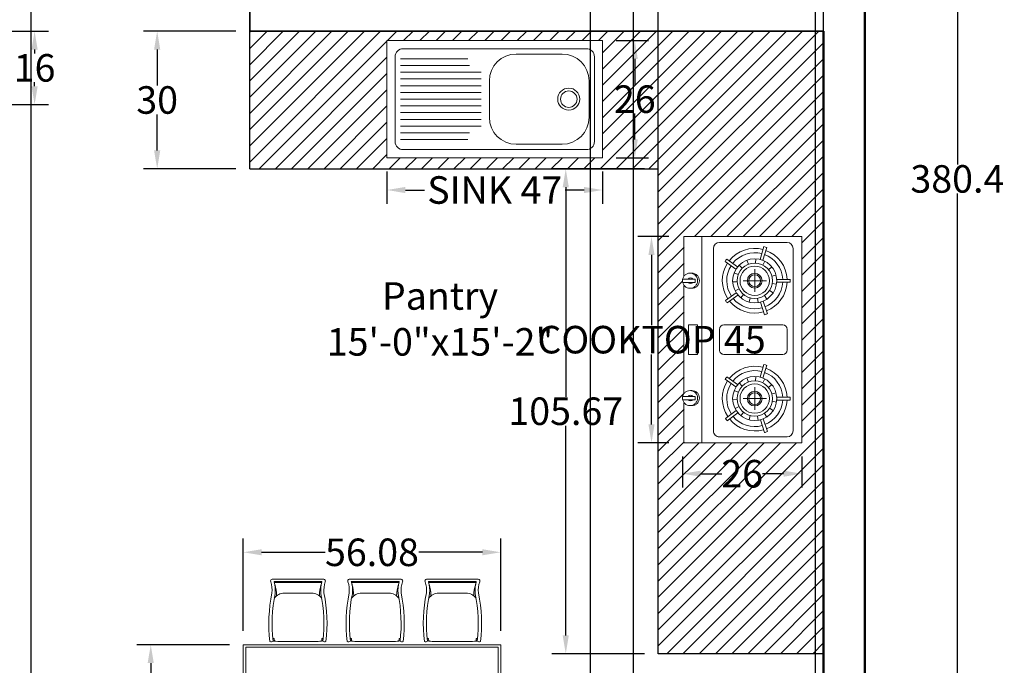
# Model space of a CAD drawing. Units: inches. Extents: x 89 to 490, y -59 to 378.
# Tile 18 of 20: x 275 to 490, y 58 to 198. Entities that reach past the tile are written whole.
import ezdxf

# ---------------------------------------------------------------- set-up
doc = ezdxf.new("R2010")
doc.units = ezdxf.units.IN
doc.header["$MEASUREMENT"] = 0
for name, color, linetype, lineweight in [('A-ANNO-DIMS', 2, 'Continuous', 18), ('A-AREA-IDEN', 7, 'Continuous', 18), ('A-FLOR-CASE', 21, 'Continuous', 25), ('A-FLOR-CASE-PATT', 25, 'Continuous', 13), ('Dining Table', 155, 'Continuous', 18), ('Gas Stove', 51, 'Continuous', 18), ('Inner Walls', 31, 'Continuous', 35), ('Outer Walls', 12, 'Continuous', 50), ('Sink', 21, 'Continuous', 18)]:
    doc.layers.add(name, color=color, linetype=linetype, lineweight=lineweight)
doc.styles.get("Standard").update_dxf_attribs({"font": 'arial.ttf'})
doc.dimstyles.get("Standard").update_dxf_attribs({"dimtxt": 6, "dimasz": 4, "dimexe": 3, "dimexo": 3, "dimgap": 0.09, "dimtad": 0, "dimtih": 1, "dimtoh": 1, "dimdec": 1, "dimzin": 0, "dimdsep": 46, "dimlunit": 3, "dimtxsty": 'Standard', "dimcen": 0.09, "dimadec": 0, "dimazin": 0, "dimtfac": 1, "dimtdec": 1, "dimtofl": 0, "dimtmove": 0, "dimatfit": 3, "dimfxl": 1, "dimtolj": 1, "dimtzin": 0, "dimarcsym": 0})

# ---------------------------------------------------------------- blocks, each defined once
blk = doc.blocks.new('A$C51F1')
at = {"color": 0}
for p, q in [((0.2273, 0.4758), (0.0436, 0.4758)), ((0.2273, 0.4676), (0.0439, 0.4676)), ((0.2273, 0.4668), (0.0439, 0.4668)), ((0.2273, 0.4758), (0.4111, 0.4758)), ((0.2273, 0.4676), (0.4107, 0.4676)), ((0.2273, 0.4668), (0.4107, 0.4668)), ((0.2273, 0.3858), (0.1205, 0.3858)), ((0.2273, 0.3858), (0.3341, 0.3858)), ((0.0417, 0.0321), (0.0321, 0.0321)), ((0.0417, 0.0321), (0.0326, 0.0278)), ((0.0435, 0.0127), (0.0417, 0.0321)), ((0.4112, 0.0127), (0.4129, 0.0321)), ((0.4129, 0.0321), (0.4225, 0.0321)), ((0.4129, 0.0321), (0.4221, 0.0278))]:
    blk.add_line(p, q, dxfattribs=at)
blk.add_lwpolyline([(0.4387, 0.4737, 0.102523), (0.4291, 0.3863, -0.080461), (0.4447, 0.0091, -0.3023), (0.4203, 0.012, 0.197932), (0.4111, 0.0127, -0.028193), (0.3571, 0.0091), (0.227, 0.0091), (0.097, 0.0091, -0.028193), (0.0429, 0.0127, 0.197932), (0.0338, 0.012, -0.3023), (0.0093, 0.0091, -0.080461), (0.0249, 0.3863, 0.102523), (0.0153, 0.4737, -0.587111), (0.0261, 0.4929), (0.4279, 0.4929, -0.587111)], format="xyb", close=True, dxfattribs=at)
for centre, radius, start, end in [((0.044, 0.4735), 0.00242, 100.34496, 201.37417), ((-0.1898, 0.4063), 0.2409, 354.55133, 15.96258), ((0.0439, 0.4669), 0.000725, 87.37617, 197.52085), ((0.0438, 0.4664), 0.000433, 71.7715, 189.22024), ((0.6445, 0.4063), 0.2409, 164.03742, 185.44867), ((0.4107, 0.4669), 0.000725, 342.47915, 92.62383), ((0.4109, 0.4664), 0.000433, 350.77976, 108.2285), ((0.4106, 0.4735), 0.00242, 338.62583, 79.65504), ((0.1214, 0.2879), 0.0978, 90.51639, 143.19267), ((-0.2563, 0.3584), 0.3173, 1.15909, 17.56409), ((0.3332, 0.2879), 0.0978, 36.80733, 89.48361), ((0.7109, 0.3584), 0.3173, 162.43591, 178.84091), ((1.1806, 0.1494), 1.1544, 168.43567, 186.83625), ((-0.7259, 0.1494), 1.1544, 353.16375, 11.56433), ((0.0397, 0.0013), 0.012, 71.75361, 116.5375), ((0.4149, 0.0013), 0.012, 63.4625, 108.24639)]:
    blk.add_arc(centre, radius, start, end, dxfattribs=at)
blk = doc.blocks.new('A$C56104318')
for p, q in [((0, 0.609), (1.12, 0.609)), ((0, 0.609), (0, 0)), ((0.084, 0.567), (1.036, 0.567)), ((1.12, 0.609), (1.12, 0)), ((0.042, 0.525), (0.042, 0.084)), ((0.42, 0.5145), (0.07, 0.5145)), ((0.672, 0.539), (0.91, 0.539)), ((1.078, 0.525), (1.078, 0.084)), ((0.07, 0.4795), (0.4294, 0.4795)), ((0.07, 0.4445), (0.49, 0.4445)), ((0.07, 0.4095), (0.49, 0.4095)), ((0.07, 0.3745), (0.49, 0.3745)), ((0.532, 0.21), (0.532, 0.399)), ((1.05, 0.399), (1.05, 0.21)), ((0.07, 0.3395), (0.49, 0.3395)), ((0.07, 0.3045), (0.49, 0.3045)), ((0.07, 0.2695), (0.49, 0.2695)), ((0.07, 0.2345), (0.49, 0.2345)), ((0.07, 0.1995), (0.49, 0.1995)), ((0.07, 0.1645), (0.4898, 0.1645)), ((0.07, 0.1295), (0.4294, 0.1295)), ((0.07, 0.0945), (0.42, 0.0945)), ((0.91, 0.07), (0.672, 0.07)), ((1.036, 0.042), (0.084, 0.042)), ((1.12, 0), (0, 0))]:
    blk.add_line(p, q)
for radius in [0.0574, 0.0427]:
    blk.add_circle((0.945, 0.3045), radius)
for centre, radius, start, end in [((0.084, 0.525), 0.042, 90, 180), ((1.036, 0.525), 0.042, 0, 90), ((0.672, 0.399), 0.14, 90, 180), ((0.91, 0.399), 0.14, 0, 90), ((0.672, 0.21), 0.14, 180, 270), ((0.91, 0.21), 0.14, 270, 0), ((0.084, 0.084), 0.042, 180, 270), ((1.036, 0.084), 0.042, 270, 0)]:
    blk.add_arc(centre, radius, start, end)
blk = doc.blocks.new('A$C559B0E78')
at = {"xscale": 729, "yscale": 729, "zscale": 729}
blk.add_blockref('A$C56104318', (0, 0), dxfattribs=at)
blk = doc.blocks.new('Gas Stove')
at = {"color": 0}
for p, q in [((732.13, 198.42), (732.13, 184.15)), ((732.13, 198.42), (757.09, 198.42)), ((757.09, 198.42), (757.09, 184.15)), ((732.84, 196.63), (732.84, 188.43)), ((733.55, 197.35), (755.66, 197.35)), ((737.3, 195.38), (737.3, 196.99)), ((737.65, 195.38), (737.65, 196.99)), ((743.36, 196.63), (745.85, 196.63)), ((751.56, 195.38), (751.56, 196.99)), ((751.92, 195.38), (751.92, 196.99)), ((756.37, 196.63), (756.37, 188.43)), ((742.82, 196.1), (742.82, 188.97)), ((746.39, 196.1), (746.39, 188.97)), ((735.79, 194.79), (736.13, 194.37)), ((736.78, 195.3), (736.92, 194.78)), ((737.89, 195.35), (737.81, 194.83)), ((738.93, 194.96), (738.64, 194.51)), ((741.48, 194.24), (739.95, 193.73)), ((750.05, 194.79), (750.39, 194.37)), ((751.05, 195.3), (751.18, 194.78)), ((752.16, 195.35), (752.07, 194.83)), ((753.19, 194.96), (752.9, 194.51)), ((755.74, 194.24), (754.21, 193.73)), ((733.34, 193.83), (734.88, 193.35)), ((733.45, 194.17), (734.98, 193.69)), ((735.09, 193.93), (735.57, 193.68)), ((737.47, 194.12), (737.47, 191.3)), ((739.72, 194.17), (739.27, 193.88)), ((740.12, 193.13), (739.59, 193.05)), ((741.59, 193.9), (740.06, 193.39)), ((747.6, 193.83), (749.14, 193.35)), ((747.71, 194.17), (749.25, 193.69)), ((749.35, 193.93), (749.83, 193.68)), ((751.74, 194.12), (751.74, 191.3)), ((753.98, 194.17), (753.53, 193.88)), ((754.38, 193.13), (753.85, 193.05)), ((755.85, 193.9), (754.33, 193.39)), ((734.8, 192.85), (735.34, 192.82)), ((734.98, 191.75), (735.48, 191.95)), ((736.06, 192.71), (738.83, 192.71)), ((740.06, 192.02), (739.54, 192.16)), ((749.07, 192.85), (749.6, 192.82)), ((749.24, 191.75), (749.74, 191.95)), ((750.36, 192.71), (753.12, 192.71)), ((754.32, 192.02), (753.8, 192.16)), ((735.58, 190.82), (735.96, 191.2)), ((736.52, 190.22), (736.71, 190.71)), ((738.69, 190.33), (738.45, 190.81)), ((739.55, 191.03), (739.14, 191.37)), ((740.16, 189.38), (739.2, 190.67)), ((749.85, 190.82), (750.22, 191.2)), ((750.78, 190.22), (750.97, 190.71)), ((752.95, 190.33), (752.71, 190.81)), ((753.82, 191.03), (753.4, 191.37)), ((754.42, 189.38), (753.47, 190.67)), ((734.84, 189.33), (735.78, 190.64)), ((735.13, 189.13), (736.07, 190.44)), ((737.61, 190.04), (737.59, 190.58)), ((739.87, 189.16), (738.92, 190.46)), ((749.11, 189.33), (750.04, 190.64)), ((749.4, 189.13), (750.33, 190.44)), ((751.88, 190.04), (751.85, 190.58)), ((754.14, 189.16), (753.18, 190.46)), ((743.36, 188.43), (745.85, 188.43)), ((733.55, 187.72), (755.66, 187.72)), ((732.13, 186.29), (757.09, 186.29)), ((737.26, 185.5), (737.69, 185.5)), ((737.26, 185.5), (737.26, 183.99)), ((737.69, 185.5), (737.69, 183.99)), ((742.82, 185.78), (742.82, 184.71)), ((742.82, 185.78), (746.39, 185.78)), ((742.82, 184.71), (746.39, 184.71)), ((746.39, 185.78), (746.39, 184.71)), ((751.47, 185.5), (751.9, 185.5)), ((751.47, 185.5), (751.47, 183.99)), ((751.9, 185.5), (751.9, 183.99)), ((732.13, 184.15), (736.91, 184.15)), ((738.03, 184.15), (751.12, 184.15)), ((752.24, 184.15), (757.09, 184.15))]:
    blk.add_line(p, q, dxfattribs=at)
for centre, radius in [((737.47, 192.71), 2.67), ((737.47, 192.71), 2.14), ((737.47, 192.71), 1.78), ((751.74, 192.71), 2.67), ((751.74, 192.71), 2.14), ((751.74, 192.71), 1.78), ((737.47, 192.71), 0.891), ((737.47, 192.71), 0.713), ((751.74, 192.71), 0.891), ((751.74, 192.71), 0.713)]:
    blk.add_circle(centre, radius, dxfattribs=at)
for centre, radius, start, end in [((733.55, 196.63), 0.713, 90, 180), ((737.47, 192.71), 3.92, 92.6053, 159.852), ((737.47, 192.71), 4.28, 87.612, 92.388), ((737.47, 192.71), 3.92, 21.0625, 87.3947), ((743.36, 196.1), 0.535, 90, 180), ((745.85, 196.1), 0.535, 0, 90), ((751.74, 192.71), 3.92, 92.6053, 159.852), ((751.74, 192.71), 4.28, 87.612, 92.388), ((751.74, 192.71), 3.92, 21.0625, 87.3947), ((755.66, 196.63), 0.713, 0, 90), ((737.47, 192.71), 3.39, 93.017, 159.4403), ((737.47, 192.71), 3.39, 21.4742, 86.983), ((751.74, 192.71), 3.39, 93.017, 159.4403), ((751.74, 192.71), 3.39, 21.4742, 86.983), ((737.47, 192.71), 4.28, 16.0692, 20.8452), ((751.74, 192.71), 4.28, 16.0692, 20.8452), ((737.47, 192.71), 4.28, 160.0692, 164.8452), ((737.47, 192.71), 3.92, 165.0625, 231.852), ((737.47, 192.71), 3.39, 165.4742, 231.4403), ((737.47, 192.71), 3.39, 309.4742, 15.4403), ((737.47, 192.71), 3.92, 309.0625, 15.852), ((751.74, 192.71), 4.28, 160.0692, 164.8452), ((751.74, 192.71), 3.92, 165.0625, 231.852), ((751.74, 192.71), 3.39, 165.4742, 231.4403), ((751.74, 192.71), 3.39, 309.4742, 15.4403), ((751.74, 192.71), 3.92, 309.0625, 15.852), ((737.47, 192.71), 3.39, 237.4742, 303.4403), ((751.74, 192.71), 3.39, 237.4742, 303.4403), ((733.55, 188.43), 0.713, 180, 270), ((737.47, 192.71), 4.28, 232.0692, 236.8452), ((737.47, 192.71), 3.92, 237.0625, 303.852), ((737.47, 192.71), 4.28, 304.0692, 308.8452), ((743.36, 188.97), 0.535, 180, 270), ((745.85, 188.97), 0.535, 270, 0), ((751.74, 192.71), 4.28, 232.0692, 236.8452), ((751.74, 192.71), 3.92, 237.0625, 303.852), ((751.74, 192.71), 4.28, 304.0692, 308.8452), ((755.66, 188.43), 0.713, 270, 0), ((737.47, 185.1), 0.916, 112.5, 135), ((737.47, 185.1), 0.916, 90, 112.5), ((737.47, 185.1), 0.916, 67.5, 90), ((737.47, 185.1), 0.916, 45, 67.5), ((751.68, 185.1), 0.916, 112.5, 135), ((751.68, 185.1), 0.916, 90, 112.5), ((751.68, 185.1), 0.916, 67.5, 90), ((751.68, 185.1), 0.916, 45, 67.5), ((737.47, 185.1), 0.916, 157.5, 180), ((737.47, 184.88), 0.916, 157.5, 180), ((737.47, 185.1), 0.916, 180, 187.0423), ((737.47, 184.88), 0.916, 180, 202.5), ((737.47, 185.1), 0.916, 135, 157.5), ((737.47, 184.88), 0.916, 135, 157.5), ((737.47, 184.88), 0.916, 112.5, 135), ((737.46, 184.94), 0.348, 124.9148, 235.0852), ((737.47, 184.88), 0.916, 90, 112.5), ((737.47, 184.88), 0.916, 67.5, 90), ((737.46, 184.94), 0.348, 311.223, 48.777), ((737.47, 184.88), 0.916, 45, 67.5), ((737.47, 185.1), 0.916, 22.5, 45), ((737.47, 184.88), 0.916, 22.5, 45), ((737.47, 185.1), 0.916, 0, 22.5), ((737.47, 184.88), 0.916, 0, 22.5), ((737.47, 184.88), 0.916, 337.5, 0), ((737.47, 185.1), 0.916, 352.9577, 0), ((751.68, 185.1), 0.916, 157.5, 180), ((751.68, 184.88), 0.916, 157.5, 180), ((751.68, 185.1), 0.916, 180, 187.0423), ((751.68, 184.88), 0.916, 180, 202.5), ((751.68, 185.1), 0.916, 135, 157.5), ((751.68, 184.88), 0.916, 135, 157.5), ((751.68, 184.88), 0.916, 112.5, 135), ((751.67, 184.94), 0.348, 124.9148, 235.0852), ((751.68, 184.88), 0.916, 90, 112.5), ((751.68, 184.88), 0.916, 67.5, 90), ((751.67, 184.94), 0.348, 311.223, 48.777), ((751.68, 184.88), 0.916, 45, 67.5), ((751.68, 185.1), 0.916, 22.5, 45), ((751.68, 184.88), 0.916, 22.5, 45), ((751.68, 185.1), 0.916, 0, 22.5), ((751.68, 184.88), 0.916, 0, 22.5), ((751.68, 184.88), 0.916, 337.5, 0), ((751.68, 185.1), 0.916, 352.9577, 0), ((737.47, 184.88), 0.916, 202.5, 225), ((737.47, 184.88), 0.916, 225, 247.5), ((737.47, 184.88), 0.916, 247.5, 270), ((737.47, 184.88), 0.916, 270, 292.5), ((737.47, 184.88), 0.916, 292.5, 315), ((737.47, 184.88), 0.916, 315, 337.5), ((751.68, 184.88), 0.916, 202.5, 225), ((751.68, 184.88), 0.916, 225, 247.5), ((751.68, 184.88), 0.916, 247.5, 270), ((751.68, 184.88), 0.916, 270, 292.5), ((751.68, 184.88), 0.916, 292.5, 315), ((751.68, 184.88), 0.916, 315, 337.5)]:
    blk.add_arc(centre, radius, start, end, dxfattribs=at)
blk = doc.blocks.new('*D42')
at = {"layer": 'A-ANNO-DIMS', "color": 0, "lineweight": -2, "transparency": 16777216}
for p, q in [((355.35, 165.16), (355.35, 158.12)), ((402.29, 165.16), (402.29, 158.12)), ((359.35, 161.12), (363.5, 161.12)), ((398.29, 161.12), (394.14, 161.12))]:
    blk.add_line(p, q, dxfattribs=at)
at = {"layer": 'A-ANNO-DIMS', "color": 0, "transparency": 16777216}
for points in [[(359.35, 161.79), (359.35, 160.45), (355.35, 161.12)], [(398.29, 161.79), (398.29, 160.45), (402.29, 161.12)]]:
    blk.add_solid(points, dxfattribs=at)
at = {"layer": 'Defpoints', "color": 0, "transparency": 16777216}
for p in [(355.35, 168.16), (402.29, 168.16), (402.29, 161.12)]:
    blk.add_point(p, dxfattribs=at)
at = {"layer": 'A-ANNO-DIMS', "color": 0, "transparency": 16777216, "insert": (378.82, 161.12), "char_height": 6, "attachment_point": 5}
blk.add_mtext('\\A1;SINK 47', dxfattribs=at)
blk = doc.blocks.new('*D43')
at = {"layer": 'A-ANNO-DIMS', "color": 0, "lineweight": -2, "transparency": 16777216}
for p, q in [((405.29, 193.68), (412.33, 193.68)), ((409.33, 189.68), (409.33, 184.07)), ((409.33, 172.16), (409.33, 177.77)), ((405.29, 168.16), (412.33, 168.16))]:
    blk.add_line(p, q, dxfattribs=at)
at = {"layer": 'A-ANNO-DIMS', "color": 0, "transparency": 16777216}
for points in [[(408.66, 189.68), (409.99, 189.68), (409.33, 193.68)], [(408.66, 172.16), (409.99, 172.16), (409.33, 168.16)]]:
    blk.add_solid(points, dxfattribs=at)
at = {"layer": 'Defpoints', "color": 0, "transparency": 16777216}
for p in [(402.29, 193.68), (409.33, 193.68), (402.29, 168.16)]:
    blk.add_point(p, dxfattribs=at)
at = {"layer": 'A-ANNO-DIMS', "color": 0, "transparency": 16777216, "insert": (409.33, 180.92), "char_height": 6, "attachment_point": 5}
blk.add_mtext('\\A1;26', dxfattribs=at)
blk = doc.blocks.new('*D44')
at = {"layer": 'A-ANNO-DIMS', "color": 0, "lineweight": -2, "transparency": 16777216}
for p, q in [((416.71, 150.97), (409.97, 150.97)), ((412.97, 146.97), (412.97, 131.7)), ((412.97, 110.04), (412.97, 125.31)), ((416.71, 106.04), (409.97, 106.04))]:
    blk.add_line(p, q, dxfattribs=at)
at = {"layer": 'A-ANNO-DIMS', "color": 0, "transparency": 16777216}
for points in [[(412.3, 146.97), (413.63, 146.97), (412.97, 150.97)], [(412.3, 110.04), (413.63, 110.04), (412.97, 106.04)]]:
    blk.add_solid(points, dxfattribs=at)
at = {"layer": 'Defpoints', "color": 0, "transparency": 16777216}
for p in [(419.71, 150.97), (412.97, 106.04), (419.71, 106.04)]:
    blk.add_point(p, dxfattribs=at)
at = {"layer": 'A-ANNO-DIMS', "color": 0, "transparency": 16777216, "insert": (412.97, 128.51), "char_height": 6, "attachment_point": 5}
blk.add_mtext('\\A1;COOKTOP 45', dxfattribs=at)
blk = doc.blocks.new('*D45')
at = {"layer": 'A-ANNO-DIMS', "color": 0, "lineweight": -2, "transparency": 16777216}
for p, q in [((419.71, 103.04), (419.71, 96.3)), ((445.72, 103.04), (445.72, 96.3)), ((423.71, 99.3), (428.28, 99.3)), ((441.72, 99.3), (437.15, 99.3))]:
    blk.add_line(p, q, dxfattribs=at)
at = {"layer": 'A-ANNO-DIMS', "color": 0, "transparency": 16777216}
for points in [[(423.71, 99.97), (423.71, 98.64), (419.71, 99.3)], [(441.72, 99.97), (441.72, 98.64), (445.72, 99.3)]]:
    blk.add_solid(points, dxfattribs=at)
at = {"layer": 'Defpoints', "color": 0, "transparency": 16777216}
for p in [(419.71, 106.04), (445.72, 106.04), (445.72, 99.3)]:
    blk.add_point(p, dxfattribs=at)
at = {"layer": 'A-ANNO-DIMS', "color": 0, "transparency": 16777216, "insert": (432.71, 99.3), "char_height": 6, "attachment_point": 5}
blk.add_mtext('\\A1;26', dxfattribs=at)
blk = doc.blocks.new('*D49')
at = {"layer": 'A-ANNO-DIMS', "color": 0, "lineweight": -2, "transparency": 16777216}
for p, q in [((462.44, 353.74), (482.59, 353.74)), ((479.59, 349.74), (479.59, 166.7)), ((479.59, -22.66), (479.59, 160.39)), ((462.44, -26.66), (482.59, -26.66))]:
    blk.add_line(p, q, dxfattribs=at)
at = {"layer": 'A-ANNO-DIMS', "color": 0, "transparency": 16777216}
for points in [[(478.92, 349.74), (480.26, 349.74), (479.59, 353.74)], [(478.92, -22.66), (480.26, -22.66), (479.59, -26.66)]]:
    blk.add_solid(points, dxfattribs=at)
at = {"layer": 'Defpoints', "color": 0, "transparency": 16777216}
for p in [(459.44, 353.74), (479.59, 353.74), (459.44, -26.66)]:
    blk.add_point(p, dxfattribs=at)
at = {"layer": 'A-ANNO-DIMS', "color": 0, "transparency": 16777216, "insert": (479.59, 163.54), "char_height": 6, "attachment_point": 5}
blk.add_mtext('\\A1;380.4', dxfattribs=at)
blk = doc.blocks.new('*D56')
at = {"layer": 'A-ANNO-DIMS', "color": 0, "lineweight": -2, "transparency": 16777216}
for p, q in [((414.44, 63.07), (414.44, 376.89)), ((450.44, 63.07), (450.44, 376.89)), ((418.44, 373.89), (428.06, 373.89)), ((446.44, 373.89), (436.82, 373.89))]:
    blk.add_line(p, q, dxfattribs=at)
at = {"layer": 'A-ANNO-DIMS', "color": 0, "transparency": 16777216}
for points in [[(418.44, 374.56), (418.44, 373.22), (414.44, 373.89)], [(446.44, 374.56), (446.44, 373.22), (450.44, 373.89)]]:
    blk.add_solid(points, dxfattribs=at)
at = {"layer": 'Defpoints', "color": 0, "transparency": 16777216}
for p in [(450.44, 373.89), (414.44, 60.07), (450.44, 60.07)]:
    blk.add_point(p, dxfattribs=at)
at = {"layer": 'A-ANNO-DIMS', "color": 0, "transparency": 16777216, "insert": (432.44, 373.89), "char_height": 6, "attachment_point": 5}
blk.add_mtext('\\A1;36', dxfattribs=at)
blk = doc.blocks.new('*D64')
at = {"layer": 'A-ANNO-DIMS', "color": 0, "lineweight": -2, "transparency": 16777216}
for p, q in [((399.65, 16.74), (399.65, 376.89)), ((450.44, 16.74), (450.44, 376.89)), ((403.65, 373.89), (414.83, 373.89)), ((446.44, 373.89), (435.27, 373.89))]:
    blk.add_line(p, q, dxfattribs=at)
at = {"layer": 'A-ANNO-DIMS', "color": 0, "transparency": 16777216}
for points in [[(403.65, 374.56), (403.65, 373.22), (399.65, 373.89)], [(446.44, 374.56), (446.44, 373.22), (450.44, 373.89)]]:
    blk.add_solid(points, dxfattribs=at)
at = {"layer": 'Defpoints', "color": 0, "transparency": 16777216}
for p in [(450.44, 373.89), (399.65, 13.74), (450.44, 13.74)]:
    blk.add_point(p, dxfattribs=at)
at = {"layer": 'A-ANNO-DIMS', "color": 0, "transparency": 16777216, "insert": (425.05, 373.89), "char_height": 6, "attachment_point": 5}
blk.add_mtext('\\A1;50.79', dxfattribs=at)
blk = doc.blocks.new('*D65')
at = {"layer": 'A-ANNO-DIMS', "color": 0, "lineweight": -2, "transparency": 16777216}
for p, q in [((322.44, 195.74), (302.29, 195.74)), ((305.29, 191.74), (305.29, 183.9)), ((305.29, 169.74), (305.29, 177.59)), ((322.44, 165.74), (302.29, 165.74))]:
    blk.add_line(p, q, dxfattribs=at)
at = {"layer": 'A-ANNO-DIMS', "color": 0, "transparency": 16777216}
for points in [[(304.62, 191.74), (305.96, 191.74), (305.29, 195.74)], [(304.62, 169.74), (305.96, 169.74), (305.29, 165.74)]]:
    blk.add_solid(points, dxfattribs=at)
at = {"layer": 'Defpoints', "color": 0, "transparency": 16777216}
for p in [(305.29, 195.74), (325.44, 195.74), (325.44, 165.74)]:
    blk.add_point(p, dxfattribs=at)
at = {"layer": 'A-ANNO-DIMS', "color": 0, "transparency": 16777216, "insert": (305.29, 180.74), "char_height": 6, "attachment_point": 5}
blk.add_mtext('\\A1;30', dxfattribs=at)
blk = doc.blocks.new('*D66')
at = {"layer": 'A-ANNO-DIMS', "color": 0, "lineweight": -2, "transparency": 16777216}
for p, q in [((411.44, 165.74), (391.29, 165.74)), ((394.29, 161.74), (394.29, 116.06)), ((394.29, 64.07), (394.29, 109.75)), ((411.44, 60.07), (391.29, 60.07))]:
    blk.add_line(p, q, dxfattribs=at)
at = {"layer": 'A-ANNO-DIMS', "color": 0, "transparency": 16777216}
for points in [[(393.62, 161.74), (394.96, 161.74), (394.29, 165.74)], [(393.62, 64.07), (394.96, 64.07), (394.29, 60.07)]]:
    blk.add_solid(points, dxfattribs=at)
at = {"layer": 'Defpoints', "color": 0, "transparency": 16777216}
for p in [(394.29, 165.74), (414.44, 165.74), (414.44, 60.07)]:
    blk.add_point(p, dxfattribs=at)
at = {"layer": 'A-ANNO-DIMS', "color": 0, "transparency": 16777216, "insert": (394.29, 112.91), "char_height": 6, "attachment_point": 5}
blk.add_mtext('\\A1;105.67', dxfattribs=at)
blk = doc.blocks.new('*D67')
at = {"layer": 'A-ANNO-DIMS', "color": 0, "lineweight": -2, "transparency": 16777216}
for p, q in [((321.04, 62.02), (300.89, 62.02)), ((303.89, 58.02), (303.89, 51.16)), ((303.89, 37.99), (303.89, 44.85)), ((321.04, 33.99), (300.89, 33.99))]:
    blk.add_line(p, q, dxfattribs=at)
at = {"layer": 'A-ANNO-DIMS', "color": 0, "transparency": 16777216}
for points in [[(303.22, 58.02), (304.56, 58.02), (303.89, 62.02)], [(303.22, 37.99), (304.56, 37.99), (303.89, 33.99)]]:
    blk.add_solid(points, dxfattribs=at)
at = {"layer": 'Defpoints', "color": 0, "transparency": 16777216}
for p in [(303.89, 62.02), (324.04, 62.02), (324.04, 33.99)]:
    blk.add_point(p, dxfattribs=at)
at = {"layer": 'A-ANNO-DIMS', "color": 0, "transparency": 16777216, "insert": (303.89, 48), "char_height": 6, "attachment_point": 5}
blk.add_mtext('\\A1;28.04', dxfattribs=at)
blk = doc.blocks.new('*D68')
at = {"layer": 'A-ANNO-DIMS', "color": 0, "lineweight": -2, "transparency": 16777216}
for p, q in [((324.04, 65.02), (324.04, 85.17)), ((380.12, 65.02), (380.12, 85.17)), ((328.04, 82.17), (341.86, 82.17)), ((376.12, 82.17), (362.3, 82.17))]:
    blk.add_line(p, q, dxfattribs=at)
at = {"layer": 'A-ANNO-DIMS', "color": 0, "transparency": 16777216}
for points in [[(328.04, 82.84), (328.04, 81.51), (324.04, 82.17)], [(376.12, 82.84), (376.12, 81.51), (380.12, 82.17)]]:
    blk.add_solid(points, dxfattribs=at)
at = {"layer": 'Defpoints', "color": 0, "transparency": 16777216}
for p in [(380.12, 82.17), (324.04, 62.02), (380.12, 62.02)]:
    blk.add_point(p, dxfattribs=at)
at = {"layer": 'A-ANNO-DIMS', "color": 0, "transparency": 16777216, "insert": (352.08, 82.17), "char_height": 6, "attachment_point": 5}
blk.add_mtext('\\A1;56.08', dxfattribs=at)
blk = doc.blocks.new('*D70')
at = {"layer": 'A-ANNO-DIMS', "color": 0, "lineweight": -2, "transparency": 16777216}
for p, q in [((261.44, 195.74), (281.59, 195.74)), ((278.59, 191.74), (278.59, 190.89)), ((278.59, 183.74), (278.59, 184.59)), ((261.44, 179.74), (281.59, 179.74))]:
    blk.add_line(p, q, dxfattribs=at)
at = {"layer": 'A-ANNO-DIMS', "color": 0, "transparency": 16777216}
for points in [[(277.92, 191.74), (279.26, 191.74), (278.59, 195.74)], [(277.92, 183.74), (279.26, 183.74), (278.59, 179.74)]]:
    blk.add_solid(points, dxfattribs=at)
at = {"layer": 'Defpoints', "color": 0, "transparency": 16777216}
for p in [(258.44, 195.74), (258.44, 179.74), (278.59, 179.74)]:
    blk.add_point(p, dxfattribs=at)
at = {"layer": 'A-ANNO-DIMS', "color": 0, "transparency": 16777216, "insert": (278.59, 187.74), "char_height": 6, "attachment_point": 5}
blk.add_mtext('\\A1;16', dxfattribs=at)
blk = doc.blocks.new('*D71')
at = {"layer": 'A-ANNO-DIMS', "color": 0, "lineweight": -2, "transparency": 16777216}
for p, q in [((409.04, 21.37), (409.04, 376.89)), ((448.72, 21.37), (448.72, 376.89)), ((413.04, 373.89), (416.35, 373.89)), ((444.72, 373.89), (441.41, 373.89))]:
    blk.add_line(p, q, dxfattribs=at)
at = {"layer": 'A-ANNO-DIMS', "color": 0, "transparency": 16777216}
for points in [[(413.04, 374.56), (413.04, 373.22), (409.04, 373.89)], [(444.72, 374.56), (444.72, 373.22), (448.72, 373.89)]]:
    blk.add_solid(points, dxfattribs=at)
at = {"layer": 'Defpoints', "color": 0, "transparency": 16777216}
for p in [(448.72, 373.89), (409.04, 18.37), (448.72, 18.37)]:
    blk.add_point(p, dxfattribs=at)
at = {"layer": 'A-ANNO-DIMS', "color": 0, "transparency": 16777216, "insert": (428.88, 373.89), "char_height": 6, "attachment_point": 5}
blk.add_mtext('\\A1;39.684', dxfattribs=at)
blk = doc.blocks.new('*D74')
at = {"layer": 'A-ANNO-DIMS', "color": 0, "lineweight": -2, "transparency": 16777216}
for p, q in [((249.44, 341.74), (249.44, -49.81)), ((277.75, 341.35), (277.75, -49.81)), ((253.44, -46.81), (253.91, -46.81)), ((273.75, -46.81), (273.28, -46.81))]:
    blk.add_line(p, q, dxfattribs=at)
at = {"layer": 'A-ANNO-DIMS', "color": 0, "transparency": 16777216}
for points in [[(253.44, -46.14), (253.44, -47.48), (249.44, -46.81)], [(273.75, -46.14), (273.75, -47.48), (277.75, -46.81)]]:
    blk.add_solid(points, dxfattribs=at)
at = {"layer": 'Defpoints', "color": 0, "transparency": 16777216}
for p in [(249.44, 344.74), (277.75, 344.35), (277.75, -46.81)]:
    blk.add_point(p, dxfattribs=at)
at = {"layer": 'A-ANNO-DIMS', "color": 0, "transparency": 16777216, "insert": (263.6, -46.81), "char_height": 6, "attachment_point": 5}
blk.add_mtext('\\A1;28.31', dxfattribs=at)

msp = doc.modelspace()

# ---------------------------------------------------------------- hatches: boundary and pattern name
at = {"layer": 'A-FLOR-CASE-PATT'}
h = msp.add_hatch(dxfattribs=at)
h.set_pattern_fill('ANSI31', color=256, scale=20)
h.set_pattern_definition([(45, (-188.7147, -85.312), (-1.767767, 1.767767), [])])
h.paths.add_polyline_path([(450.4414, 195.7413), (325.4414, 195.7413), (325.4414, 165.7413), (414.4414, 165.7413), (414.4414, 60.0723), (450.4414, 60.0723)])
h.paths.add_polyline_path([(445.7222, 150.9692), (445.7222, 106.0431), (420.0501, 106.0431), (420.0501, 114.769, -0.06610496), (419.8327, 115.1447, -0.0984914), (419.7072, 115.7756, -0.0984914), (419.8327, 116.4065, -0.06610496), (420.0501, 116.7822), (420.0501, 140.3496, -0.06610496), (419.8327, 140.7253, -0.0984914), (419.7072, 141.3562, -0.0984914), (419.8327, 141.9871, -0.06610496), (420.0501, 142.3627), (420.0501, 150.9692)], flags=16)
h.paths.add_polyline_path([(442.5132, 149.6856, -0.41420943), (443.7968, 148.402), (443.7968, 108.6103, -0.4142177), (442.5132, 107.3267), (427.7518, 107.3267, -0.41421356), (426.4682, 108.6103), (426.4682, 148.402, -0.41421356), (427.7518, 149.6856)], flags=0)
h.paths.add_polyline_path([(438.0787, 148.5825), (437.8851, 147.97, -0.30214028), (442.5059, 141.6631), (443.1483, 141.6631, -0.02084238), (443.1483, 141.0213), (442.5059, 141.0213, -0.29779118), (437.9906, 134.754), (438.194, 134.1447, -0.02084238), (437.5852, 133.9415), (437.3818, 134.5508, -0.29996443), (429.9717, 136.8933), (429.455, 136.5116, -0.02084238), (429.0737, 137.0278), (429.5903, 137.4095, -0.29996443), (429.5283, 145.1808), (429.0056, 145.5542, -0.02084238), (429.3787, 146.0764), (429.9014, 145.703, -0.29996443), (437.2732, 148.1634), (437.4668, 148.7759, -0.02084238)], flags=0)
h.paths.add_polyline_path([(440.2669, 141.3422, -1), (430.6399, 141.3422, -1)], flags=0)
h.paths.add_polyline_path([(439.3042, 141.3422, -1), (431.6026, 141.3422, -1)], flags=0)
h.paths.add_polyline_path([(438.6624, 141.3422, -1), (432.2444, 141.3422, -1)], flags=0)
h.paths.add_polyline_path([(437.0579, 141.3422, -1), (433.8489, 141.3422, -1)], flags=0)
h.paths.add_polyline_path([(436.737, 141.3422, -1), (434.1698, 141.3422, -1)], flags=0)
h.paths.add_polyline_path([(402.2862, 168.1597), (355.3485, 168.1597), (355.3485, 193.6821), (402.2862, 193.6821)], flags=16)
h.paths.add_polyline_path([(422.3911, 142.8794, -0.0984914), (422.9259, 142.522, -0.0984914), (423.2833, 141.9871, -0.0984914), (423.4088, 141.3562, -0.0984914), (423.2833, 140.7253, -0.0984914), (422.9259, 140.1904, -0.0984914), (422.3911, 139.833, -0.1296214), (421.558, 139.7199, 0.06754933), (421.9868, 139.833, 0.0984914), (422.5217, 140.1904, 0.0984914), (422.879, 140.7253, 0.0984914), (423.0045, 141.3562, 0.0984914), (422.879, 141.9871, 0.0984914), (422.5217, 142.522, 0.0984914), (421.9868, 142.8794, 0.06754933), (421.558, 142.9924, -0.1296214)], flags=0)
h.paths.add_polyline_path([(422.4695, 141.7273), (422.4695, 140.9571), (421.9407, 140.9571, -0.45337861), (420.9998, 140.9571), (422.4695, 140.9571), (422.4695, 141.7273), (420.9574, 141.7273, -0.52151233), (421.9832, 141.7273)], flags=0)
h.paths.add_polyline_path([(400.5261, 171.6885, -0.41563499), (398.7659, 169.9198), (358.8688, 169.9198, -0.41421379), (357.1087, 171.68), (357.1087, 190.1617, -0.41279405), (358.8603, 191.9219), (398.7574, 191.9219, -0.41421356), (400.5261, 190.1703)], flags=0)
h.paths.add_polyline_path([(399.3527, 176.9605, -0.41421356), (393.4854, 171.0933), (393.4854, 171.0933), (383.5112, 171.0933, -0.41421356), (377.6439, 176.9605), (377.6439, 176.9605), (377.6439, 184.8812, -0.41334382), (383.4937, 190.7484), (393.468, 190.7484, -0.41508384), (399.3527, 184.8812)], flags=0)
h.paths.add_polyline_path([(392.5465, 180.9208, -1), (397.358, 180.9208, -1)], flags=0)
h.paths.add_polyline_path([(393.1618, 180.9208, -1), (396.7427, 180.9208, -1)], flags=0)
h.paths.add_polyline_path([(441.5505, 131.7152, -0.41421356), (442.5132, 130.7525), (442.5132, 126.2598, -0.41421356), (441.5505, 125.2971), (428.7145, 125.2971, -0.4142077), (427.7518, 126.2598), (427.7518, 130.7524, -0.41421942), (428.7145, 131.7152)], flags=0)
h.paths.add_polyline_path([(422.9731, 131.7152), (422.9731, 125.2971), (421.0477, 125.2971), (421.0477, 131.7152)], flags=0)
h.paths.add_polyline_path([(438.0787, 122.9104), (437.8851, 122.2979, -0.30214028), (442.5059, 115.991), (443.1483, 115.991, -0.02084238), (443.1483, 115.3492), (442.5059, 115.3492, -0.29779118), (437.9906, 109.082), (438.194, 108.4726, -0.02084238), (437.5852, 108.2694), (437.3818, 108.8788, -0.29996443), (429.9717, 111.2213), (429.455, 110.8395, -0.02084238), (429.0737, 111.3557), (429.5903, 111.7375, -0.29996443), (429.5283, 119.5087), (429.0056, 119.8822, -0.02084238), (429.3787, 120.4044), (429.9014, 120.0309, -0.29996443), (437.2732, 122.4914), (437.4668, 123.1039, -0.02084238)], flags=0)
h.paths.add_polyline_path([(440.2669, 115.6701, -1), (430.6399, 115.6701, -1)], flags=0)
h.paths.add_polyline_path([(439.3042, 115.6701, -1), (431.6026, 115.6701, -1)], flags=0)
h.paths.add_polyline_path([(438.6624, 115.6701, -1), (432.2444, 115.6701, -1)], flags=0)
h.paths.add_polyline_path([(437.0579, 115.6701, -1), (433.8489, 115.6701, -1)], flags=0)
h.paths.add_polyline_path([(436.737, 115.6701, -1), (434.1698, 115.6701, -1)], flags=0)
h.paths.add_polyline_path([(422.3911, 117.2988, -0.0984914), (422.9259, 116.9414, -0.0984914), (423.2833, 116.4065, -0.0984914), (423.4088, 115.7756, -0.0984914), (423.2833, 115.1447, -0.0984914), (422.9259, 114.6098, -0.0984914), (422.3911, 114.2524, -0.1296214), (421.558, 114.1394, 0.06754933), (421.9868, 114.2524, 0.0984914), (422.5217, 114.6098, 0.0984914), (422.879, 115.1447, 0.0984914), (423.0045, 115.7756, 0.0984914), (422.879, 116.4065, 0.0984914), (422.5217, 116.9414, 0.0984914), (421.9868, 117.2988, 0.06754933), (421.558, 117.4118, -0.1296214)], flags=0)
h.paths.add_polyline_path([(421.9832, 116.1467), (422.4695, 116.1467), (422.4695, 115.3765), (421.9407, 115.3765, -0.45337861), (420.9998, 115.3765), (422.4695, 115.3765), (422.4695, 116.1467), (420.9574, 116.1467, -0.52151233)], flags=0)

# ---------------------------------------------------------------- linework, layer by layer
at = {"layer": 'A-FLOR-CASE'}
for p, q in [((325.4414, 165.7413), (325.4414, 195.7413)), ((325.4414, 165.7413), (414.4414, 165.7413)), ((414.4414, 60.0723), (414.4414, 165.7413)), ((450.4414, 60.0723), (414.4414, 60.0723))]:
    msp.add_line(p, q, dxfattribs=at)
at = {"layer": 'Dining Table', "ltscale": 0.5}
for points in [[(324.0409, 33.9856), (380.116, 33.9856), (380.116, 62.0232), (324.0409, 62.0232)], [(324.6016, 34.5464), (379.5552, 34.5464), (379.5552, 61.4624), (324.6016, 61.4624)]]:
    msp.add_lwpolyline(points, close=True, dxfattribs=at)
at = {"layer": 'Inner Walls'}
for q in [(325.4414, 206.7413), (450.4414, 195.7413)]:
    msp.add_line((325.4414, 195.7413), q, dxfattribs=at)
at = {"layer": 'Outer Walls'}
msp.add_line((450.4414, 13.7413), (450.4414, 195.7413), dxfattribs=at)
msp.add_lwpolyline([(214.6478, 67.7413), (265.4414, 67.7413), (265.4414, 4.7413), (459.4414, 4.7413), (459.4414, 353.7413), (127.4414, 353.7413), (127.4414, 13.7413)], dxfattribs=at)

# ---------------------------------------------------------------- block references
at = {"layer": 'Dining Table', "ltscale": 0.5, "yscale": 28.0375393373698, "zscale": 28.0375393373698}
for p, xscale in [((329.592, 62.4687), 28.0375393373698), ((346.4145, 62.4687), 28.0375393373698), ((375.9667, 62.4687), -28.0375393373698)]:
    msp.add_blockref('A$C51F1', p, dxfattribs=dict(at, xscale=xscale))
at = {"layer": 'Gas Stove', "xscale": 1.799839398615028, "yscale": 1.799839398615028, "zscale": 1.799839398615028, "rotation": 270}
msp.add_blockref('Gas Stove', (88.6022, 1468.6771), dxfattribs=at)
at = {"layer": 'Sink', "xscale": 0.0574878350584968, "yscale": 0.0574878350584968, "zscale": 0.0574878350584968}
msp.add_blockref('A$C559B0E78', (355.3485, 168.1597), dxfattribs=at)

# ---------------------------------------------------------------- texts
at = {"layer": 'A-AREA-IDEN', "insert": (343.7032, 141.031), "char_height": 6, "attachment_point": 1}
msp.add_mtext_dynamic_manual_height_columns('\\pxqc;Pantry\\P15\'-0"x15\'-2"', width=46.403971, gutter_width=1, heights=[0], dxfattribs=at)

# ---------------------------------------------------------------- dimensions: what is measured, and where the dimension line sits
at = {"layer": 'A-ANNO-DIMS'}
for base, p1, p2, override, picture, middle in [((450.4414, 373.8913), (399.6539, 13.7413), (450.4414, 13.7413), {"dimdec": 2, "dimlfac": 1, "dimrnd": 0, "dimzin": 0, "dimdsep": 46, "dimlunit": 2}, '*D64', (425.0477, 373.8913)), ((448.7229, 373.8913), (409.0388, 18.3742), (448.7229, 18.3742), {"dimdec": 3, "dimlfac": 1, "dimrnd": 0, "dimzin": 0, "dimdsep": 46, "dimlunit": 2}, '*D71', (428.8809, 373.8913)), ((450.4414, 373.8913), (414.4414, 60.0723), (450.4414, 60.0723), {"dimdec": 0, "dimlfac": 1, "dimrnd": 0, "dimzin": 0, "dimdsep": 46, "dimlunit": 2}, '*D56', (432.4414, 373.8913)), ((277.7535, -46.8094), (249.4414, 344.7413), (277.7535, 344.3468), {"dimdec": 2, "dimlfac": 1, "dimrnd": 0, "dimzin": 0, "dimdsep": 46, "dimlunit": 2}, '*D74', (263.5974, -46.8094)), ((445.7222, 99.3042), (419.7072, 106.0431), (445.7222, 106.0431), {"dimdec": 0, "dimlfac": 1, "dimrnd": 0, "dimzin": 0, "dimdsep": 46, "dimlunit": 2}, '*D45', (432.7147, 99.3042)), ((380.116, 82.1732), (324.0409, 62.0232), (380.116, 62.0232), {"dimdec": 2, "dimlfac": 1, "dimrnd": 0, "dimzin": 0, "dimdsep": 46, "dimlunit": 2}, '*D68', (352.0784, 82.1732))]:
    dim = msp.add_linear_dim(base=base, p1=p1, p2=p2, dimstyle='Standard', override=override, dxfattribs=at)
    dim.commit()
    dim.dimension.update_dxf_attribs({"geometry": picture, "text_midpoint": middle})
for base, p1, p2, angle, override, picture, middle in [((479.5914, 353.7413), (459.4414, -26.6594), (459.4414, 353.7413), 90, {"dimdec": 1, "dimlfac": 1, "dimrnd": 0, "dimzin": 0, "dimdsep": 46, "dimlunit": 2}, '*D49', (479.5914, 163.5409)), ((278.5914, 179.7413), (258.4414, 195.7413), (258.4414, 179.7413), 270, {"dimdec": 0, "dimlfac": 1, "dimrnd": 0, "dimzin": 0, "dimdsep": 46, "dimlunit": 2}, '*D70', (278.5914, 187.7413)), ((305.2914, 195.7413), (325.4414, 165.7413), (325.4414, 195.7413), 90, {"dimdec": 0, "dimlfac": 1, "dimrnd": 0, "dimzin": 0, "dimdsep": 46, "dimlunit": 2}, '*D65', (305.2914, 180.7413)), ((409.3269, 193.6821), (402.2862, 168.1597), (402.2862, 193.6821), 90, {"dimdec": 0, "dimlfac": 1, "dimrnd": 0, "dimzin": 0, "dimdsep": 46, "dimlunit": 2}, '*D43', (409.3269, 180.9209)), ((394.2914, 165.7413), (414.4414, 60.0723), (414.4414, 165.7413), 90, {"dimdec": 2, "dimlfac": 1, "dimrnd": 0, "dimzin": 0, "dimdsep": 46, "dimlunit": 2}, '*D66', (394.2914, 112.9068)), ((303.8909, 62.0232), (324.0409, 33.9856), (324.0409, 62.0232), 90, {"dimdec": 2, "dimlfac": 1, "dimrnd": 0, "dimzin": 0, "dimdsep": 46, "dimlunit": 2}, '*D67', (303.8909, 48.0044))]:
    dim = msp.add_linear_dim(base=base, p1=p1, p2=p2, angle=angle, dimstyle='Standard', override=override, dxfattribs=at)
    dim.commit()
    dim.dimension.update_dxf_attribs({"geometry": picture, "text_midpoint": middle})
dim = msp.add_linear_dim(base=(402.2862, 161.119), p1=(355.3485, 168.1597), p2=(402.2862, 168.1597), text='SINK <>', dimstyle='Standard', override={"dimdec": 0, "dimlfac": 1, "dimrnd": 0, "dimzin": 0, "dimdsep": 46, "dimlunit": 2}, dxfattribs=at)
dim.commit()
dim.dimension.update_dxf_attribs({"geometry": '*D42', "text_midpoint": (378.8174, 161.119)})
dim = msp.add_linear_dim(base=(412.9683, 106.0431), p1=(419.7072, 150.9692), p2=(419.7072, 106.0431), angle=270, text='COOKTOP <>', dimstyle='Standard', override={"dimdec": 0, "dimlfac": 1, "dimrnd": 0, "dimzin": 0, "dimdsep": 46, "dimlunit": 2}, dxfattribs=at)
dim.commit()
dim.dimension.update_dxf_attribs({"geometry": '*D44', "text_midpoint": (412.9683, 128.5061)})

doc.saveas('drawing.dxf')
